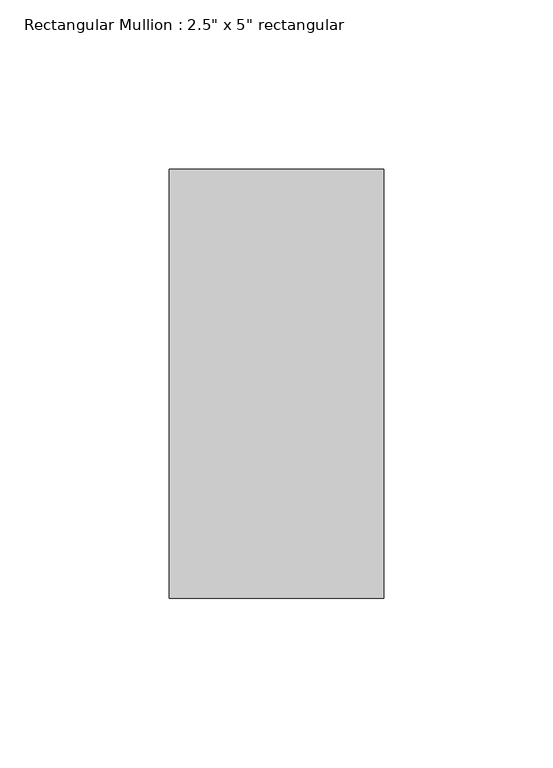
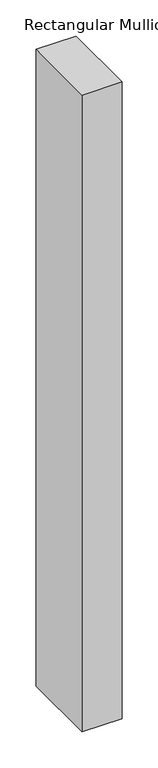
"""IFC4 building model written with IfcOpenShell, lengths in millimetres: member geometry."""

from ifc_helpers import new_model, si_unit, frame, origin, place, context, project, spatial, polyline, outline, extrude, source, transform, mapped, element, save


def member_0d004d8a(model_context):
    return source(origin(), model_context, "Body", "SweptSolid", [
        extrude(outline(polyline([(0.0, 63.5), (0.0, -63.5), (-63.5, -63.5), (-63.5, 63.5), (0.0, 63.5)])), frame((0.0, 0.0, -1073.1500002), z_axis=(0.0, 0.0, 1.0), x_axis=(1.0, 0.0, 0.0)), (0.0, 0.0, 1.0), 1073.1500002),
    ])


if __name__ == "__main__":
    model = new_model("IFC4")
    model_context = context("Model", 3, world=origin())
    ifc_project = project(units=[si_unit("LENGTHUNIT", "METRE", prefix="MILLI")], contexts=[model_context])
    site = spatial("IfcSite", under=ifc_project)
    building = spatial("IfcBuilding", under=site)
    placement = place(None, origin())
    member_shape = member_0d004d8a(model_context)
    element("IfcMember", 1, ObjectType="Rectangular Mullion : 2.5\" x 5\" rectangular", at=placement, inside=building, context=model_context, shape_type="MappedRepresentation", body=[
        mapped(member_shape, transform((0.0, 0.0, 0.0), x_axis=(1.0, 0.0, 0.0), y_axis=(0.0, 1.0, 0.0), z_axis=(0.0, 0.0, 1.0))),
    ])
    save(model, "model.ifc")

# Revit data of these elements
# Type "Rectangular Mullion : 2.5\" x 5\" rectangular"
#   built-in parameter 1007304 = 0.416667 (stored number, unit not read)
#   built-in parameter 1007301 = 0.104167 (stored number, unit not read)
#   built-in parameter 1007300 = 0.104167 (stored number, unit not read)
# Element 1 (IfcMember, "Rectangular Mullion : 2.5\" x 5\" rectangular")
#   Materials on its faces: "Aluminum"
# Materials
#   "Aluminum": class "Metal", colour RGB 247 247 247, transparency 0, Description = "Aluminum 6061", Cost = 0
